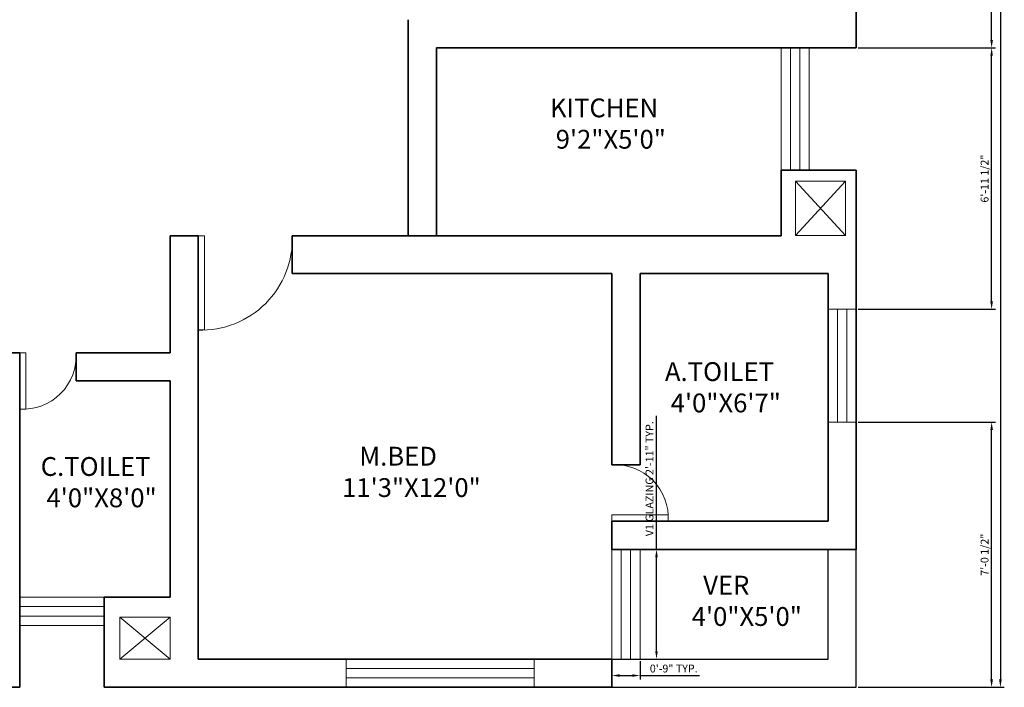
# Model space of a CAD drawing. Units: inches. Extents: x 3941 to 4852, y 2755 to 3388.
# Tile 4 of 5: x 4537 to 4852, y 2800 to 3013. Entities that reach past the tile are written whole.
import ezdxf

# ---------------------------------------------------------------- set-up
doc = ezdxf.new("R2010")
doc.units = ezdxf.units.IN
for name, color, linetype, lineweight in [('A-ANNO-DIMS', 2, 'Continuous', 18), ('A-AREA-IDEN', 7, 'Continuous', 18), ('A-DOOR', 2, 'Continuous', 18), ('A-FLOR-OPEN', 7, 'Continuous', 18), ('A-GLAZ', 5, 'Continuous', 18), ('A-WALL', 7, 'Continuous', 35), ('A-WALL-PRPT', 6, 'Continuous', 25)]:
    doc.layers.add(name, color=color, linetype=linetype, lineweight=lineweight)
doc.styles.get("Standard").update_dxf_attribs({"font": 'arial.ttf'})
doc.dimstyles.new('ISO-25', dxfattribs={"dimtxt": 2.5, "dimasz": 2.5, "dimexe": 1.25, "dimexo": 0.625, "dimtad": 1, "dimlunit": 3, "dimtxsty": 'Standard', "dimcen": 2.5, "dimadec": 0, "dimazin": 0, "dimtfac": 1, "dimtmove": 0, "dimatfit": 3, "dimfxl": 1, "dimarcsym": 0})

# ---------------------------------------------------------------- blocks, each defined once
blk = doc.blocks.new('*D2')
at = {"layer": 'A-ANNO-DIMS', "color": 0, "lineweight": -2, "transparency": 16777216}
for p, q in [((4804.88, 3327.75), (4851.51, 3327.75)), ((4850.26, 3325.25), (4850.26, 2802.25)), ((4804.88, 2799.75), (4851.51, 2799.75))]:
    blk.add_line(p, q, dxfattribs=at)
at = {"layer": 'A-ANNO-DIMS', "color": 0, "transparency": 16777216}
for points in [[(4849.85, 3325.25), (4850.68, 3325.25), (4850.26, 3327.75)], [(4849.85, 2802.25), (4850.68, 2802.25), (4850.26, 2799.75)]]:
    blk.add_solid(points, dxfattribs=at)
at = {"layer": 'Defpoints', "color": 0, "transparency": 16777216}
for p in [(4804.25, 3327.75), (4804.25, 2799.75), (4850.26, 2799.75)]:
    blk.add_point(p, dxfattribs=at)
at = {"layer": 'A-ANNO-DIMS', "color": 0, "transparency": 16777216, "insert": (4846.59, 3063.75), "char_height": 6, "attachment_point": 5, "rotation": 90}
blk.add_mtext('44\'-5"', dxfattribs=at)
blk = doc.blocks.new('WINDOW-60IN')
for p, q in [((0, 60), (9, 60)), ((0, 60), (0, 0)), ((3, 60), (3, 0)), ((6, 60), (6, 0)), ((9, 0), (9, 60)), ((0, 0), (9, 0))]:
    blk.add_line(p, q)
blk = doc.blocks.new('WINDOW-27IN')
for p, q in [((0, 0), (0, 27)), ((0, 27), (9, 27)), ((3, 0), (3, 27)), ((6, 0), (6, 27)), ((9, 27), (9, 0)), ((9, 0), (0, 0))]:
    blk.add_line(p, q)
blk = doc.blocks.new('WINDOW-36IN')
for p, q in [((0, 36), (9, 36)), ((0, 36), (0, 0)), ((3, 0), (3, 36)), ((6, 0), (6, 36)), ((9, 0), (9, 36)), ((0, 0), (9, 0))]:
    blk.add_line(p, q)
blk = doc.blocks.new('VERANDA-GLAZING-35IN')
for p, q in [((0, 35), (0, 0)), ((0, 35), (9, 35)), ((3, 35), (3, 0)), ((6, 35), (6, 0)), ((9, 35), (9, 0)), ((9, 35), (9, 0)), ((9, 0), (0, 0))]:
    blk.add_line(p, q)
blk = doc.blocks.new('DOOR-SWING-18IN')
for p, q in [((0.03, 0), (0.03, 2)), ((0.03, 2), (18.03, 2)), ((18.03, 0), (0.03, 0)), ((18.03, 2), (18.03, 0))]:
    blk.add_line(p, q)
blk.add_arc((17.03, 1), 17.03, 86.6335, 183.3665)
blk = doc.blocks.new('DOOR-SWING-30IN')
for p, q in [((0, 30.02), (30, 30.02)), ((0, 28.02), (0, 30.02)), ((30, 30.02), (30, 28.02)), ((30, 28.02), (0, 28.02))]:
    blk.add_line(p, q)
blk.add_arc((1, 29.02), 29.02, 268.0251, 1.9749)
blk = doc.blocks.new('*D25')
at = {"layer": 'A-ANNO-DIMS', "color": 0, "lineweight": -2, "transparency": 16777216}
for p, q in [((4740.5, 2843.75), (4740.5, 2886.36)), ((4735.88, 2843.75), (4741.75, 2843.75)), ((4740.5, 2811.25), (4740.5, 2841.25)), ((4735.88, 2808.75), (4741.75, 2808.75))]:
    blk.add_line(p, q, dxfattribs=at)
at = {"layer": 'A-ANNO-DIMS', "color": 0, "transparency": 16777216}
for points in [[(4740.09, 2841.25), (4740.92, 2841.25), (4740.5, 2843.75)], [(4740.09, 2811.25), (4740.92, 2811.25), (4740.5, 2808.75)]]:
    blk.add_solid(points, dxfattribs=at)
at = {"layer": 'Defpoints', "color": 0, "transparency": 16777216}
for p in [(4735.25, 2843.75), (4740.5, 2843.75), (4735.25, 2808.75)]:
    blk.add_point(p, dxfattribs=at)
at = {"layer": 'A-ANNO-DIMS', "color": 0, "transparency": 16777216, "insert": (4738.59, 2866.31), "char_height": 2.5, "attachment_point": 5, "rotation": 90}
blk.add_mtext('V1 GLAZING 2\'-11" TYP.', dxfattribs=at)
blk = doc.blocks.new('*D26')
at = {"layer": 'A-ANNO-DIMS', "color": 0, "lineweight": -2, "transparency": 16777216}
for p, q in [((4726.25, 2808.13), (4726.25, 2802.25)), ((4735.25, 2808.13), (4735.25, 2802.25)), ((4728.75, 2803.5), (4732.75, 2803.5)), ((4735.25, 2803.5), (4754.24, 2803.5))]:
    blk.add_line(p, q, dxfattribs=at)
at = {"layer": 'A-ANNO-DIMS', "color": 0, "transparency": 16777216}
for points in [[(4728.75, 2803.92), (4728.75, 2803.09), (4726.25, 2803.5)], [(4732.75, 2803.92), (4732.75, 2803.09), (4735.25, 2803.5)]]:
    blk.add_solid(points, dxfattribs=at)
at = {"layer": 'Defpoints', "color": 0, "transparency": 16777216}
for p in [(4726.25, 2808.75), (4735.25, 2808.75), (4735.25, 2803.5)]:
    blk.add_point(p, dxfattribs=at)
at = {"layer": 'A-ANNO-DIMS', "color": 0, "transparency": 16777216, "insert": (4746, 2805.41), "char_height": 2.5, "attachment_point": 5}
blk.add_mtext('0\'-9" TYP.', dxfattribs=at)
blk = doc.blocks.new('*D30')
at = {"layer": 'A-ANNO-DIMS', "color": 0, "lineweight": -2, "transparency": 16777216}
for p, q in [((4804.88, 2884.36), (4848.72, 2884.36)), ((4847.47, 2802.25), (4847.47, 2881.86)), ((4804.88, 2799.75), (4848.72, 2799.75))]:
    blk.add_line(p, q, dxfattribs=at)
at = {"layer": 'A-ANNO-DIMS', "color": 0, "transparency": 16777216}
for points in [[(4847.05, 2881.86), (4847.88, 2881.86), (4847.47, 2884.36)], [(4847.05, 2802.25), (4847.88, 2802.25), (4847.47, 2799.75)]]:
    blk.add_solid(points, dxfattribs=at)
at = {"layer": 'Defpoints', "color": 0, "transparency": 16777216}
for p in [(4804.25, 2884.36), (4847.47, 2884.36), (4804.25, 2799.75)]:
    blk.add_point(p, dxfattribs=at)
at = {"layer": 'A-ANNO-DIMS', "color": 0, "transparency": 16777216, "insert": (4845.55, 2842.06), "char_height": 2.5, "attachment_point": 5, "rotation": 90}
blk.add_mtext('7\'-0 1/2"', dxfattribs=at)
blk = doc.blocks.new('*D31')
at = {"layer": 'A-ANNO-DIMS', "color": 0, "lineweight": -2, "transparency": 16777216}
for p, q in [((4804.88, 3003.75), (4848.72, 3003.75)), ((4847.47, 2922.86), (4847.47, 3001.25)), ((4804.88, 2920.36), (4848.72, 2920.36))]:
    blk.add_line(p, q, dxfattribs=at)
at = {"layer": 'A-ANNO-DIMS', "color": 0, "transparency": 16777216}
for points in [[(4847.05, 3001.25), (4847.88, 3001.25), (4847.47, 3003.75)], [(4847.05, 2922.86), (4847.88, 2922.86), (4847.47, 2920.36)]]:
    blk.add_solid(points, dxfattribs=at)
at = {"layer": 'Defpoints', "color": 0, "transparency": 16777216}
for p in [(4804.25, 3003.75), (4847.47, 3003.75), (4804.25, 2920.36)]:
    blk.add_point(p, dxfattribs=at)
at = {"layer": 'A-ANNO-DIMS', "color": 0, "transparency": 16777216, "insert": (4845.55, 2962.06), "char_height": 2.5, "attachment_point": 5, "rotation": 90}
blk.add_mtext('6\'-11 1/2"', dxfattribs=at)
blk = doc.blocks.new('*D32')
at = {"layer": 'A-ANNO-DIMS', "color": 0, "lineweight": -2, "transparency": 16777216}
for p, q in [((4804.88, 3044.64), (4848.72, 3044.64)), ((4847.47, 3006.25), (4847.47, 3042.14)), ((4804.88, 3003.75), (4848.72, 3003.75))]:
    blk.add_line(p, q, dxfattribs=at)
at = {"layer": 'A-ANNO-DIMS', "color": 0, "transparency": 16777216}
for points in [[(4847.05, 3042.14), (4847.88, 3042.14), (4847.47, 3044.64)], [(4847.05, 3006.25), (4847.88, 3006.25), (4847.47, 3003.75)]]:
    blk.add_solid(points, dxfattribs=at)
at = {"layer": 'Defpoints', "color": 0, "transparency": 16777216}
for p in [(4804.25, 3044.64), (4847.47, 3044.64), (4804.25, 3003.75)]:
    blk.add_point(p, dxfattribs=at)
at = {"layer": 'A-ANNO-DIMS', "color": 0, "transparency": 16777216, "insert": (4845.56, 3024.2), "char_height": 2.5, "attachment_point": 5, "rotation": 90}
blk.add_mtext('3\'-5"', dxfattribs=at)

msp = doc.modelspace()

# ---------------------------------------------------------------- linework, layer by layer
at = {"layer": 'A-FLOR-OPEN'}
for p, q in [((4800.843, 2961.285), (4784.843, 2961.285)), ((4784.843, 2961.285), (4784.843, 2943.934)), ((4784.843, 2943.934), (4800.843, 2961.285)), ((4784.843, 2961.285), (4800.843, 2943.934)), ((4800.843, 2943.934), (4800.843, 2961.285)), ((4784.843, 2943.934), (4800.843, 2943.934)), ((4585.254, 2822.116), (4569.254, 2822.116)), ((4569.254, 2822.116), (4569.254, 2808.754)), ((4569.254, 2808.754), (4585.254, 2822.116)), ((4569.254, 2822.116), (4585.254, 2808.754)), ((4585.254, 2808.754), (4585.254, 2822.116)), ((4569.254, 2808.754), (4585.254, 2808.754))]:
    msp.add_line(p, q, dxfattribs=at)
at = {"layer": 'A-GLAZ'}
for p, q in [((4780.254, 3003.754), (4780.254, 2964.754)), ((4789.254, 3003.754), (4780.254, 3003.754)), ((4783.254, 3003.754), (4783.254, 2964.754)), ((4786.254, 3003.754), (4786.254, 2964.754)), ((4789.254, 2964.754), (4789.254, 3003.754)), ((4780.254, 2964.754), (4789.254, 2964.754))]:
    msp.add_line(p, q, dxfattribs=at)
at = {"layer": 'A-WALL'}
for p, q in [((4804.254, 3003.754), (4804.254, 3132.754)), ((4661.254, 3012.754), (4661.254, 2943.754)), ((4804.254, 3003.754), (4670.254, 3003.754)), ((4670.254, 3003.754), (4670.254, 2943.754)), ((4804.254, 2964.754), (4780.254, 2964.754)), ((4780.254, 2964.754), (4780.254, 2943.754)), ((4804.254, 2943.754), (4804.254, 2964.754)), ((4585.254, 2931.754), (4585.254, 2943.754)), ((4585.254, 2943.754), (4594.254, 2943.754)), ((4594.254, 2943.754), (4594.254, 2897.492)), ((4780.254, 2943.754), (4624.254, 2943.754)), ((4624.254, 2943.754), (4624.254, 2931.754)), ((4804.254, 2843.754), (4804.254, 2943.754)), ((4585.254, 2931.754), (4585.254, 2906.492)), ((4624.254, 2931.754), (4726.254, 2931.754)), ((4726.254, 2870.754), (4726.254, 2931.754)), ((4735.254, 2931.754), (4795.254, 2931.754)), ((4735.254, 2870.754), (4735.254, 2931.754)), ((4795.254, 2852.754), (4795.254, 2931.754)), ((4528.254, 2906.492), (4537.254, 2906.492)), ((4537.254, 2906.492), (4537.254, 2897.492)), ((4585.254, 2906.492), (4555.254, 2906.492)), ((4555.254, 2906.492), (4555.254, 2897.492)), ((4537.254, 2799.754), (4537.254, 2897.492)), ((4585.254, 2897.492), (4555.254, 2897.492)), ((4585.254, 2828.492), (4585.254, 2897.492)), ((4594.254, 2808.754), (4594.254, 2897.492)), ((4726.254, 2870.754), (4735.254, 2870.754)), ((4726.254, 2852.754), (4795.254, 2852.754)), ((4726.254, 2843.754), (4726.254, 2852.754)), ((4726.254, 2843.754), (4804.254, 2843.754)), ((4585.254, 2828.492), (4564.254, 2828.492)), ((4564.254, 2828.492), (4564.254, 2799.754)), ((4726.254, 2808.754), (4594.254, 2808.754)), ((4726.254, 2799.754), (4726.254, 2808.754)), ((4537.254, 2799.754), (4246.254, 2799.754)), ((4564.254, 2799.754), (4585.254, 2799.754)), ((4726.254, 2799.754), (4585.254, 2799.754))]:
    msp.add_line(p, q, dxfattribs=at)
at = {"layer": 'A-WALL-PRPT'}
for p, q in [((4795.254, 2808.754), (4795.254, 2843.754)), ((4804.254, 2799.754), (4804.254, 2843.754)), ((4726.254, 2808.754), (4795.254, 2808.754)), ((4726.254, 2799.754), (4804.254, 2799.754))]:
    msp.add_line(p, q, dxfattribs=at)

# ---------------------------------------------------------------- block references
at = {"layer": 'A-DOOR', "extrusion": (0, 0, -1), "zscale": -1}
for name, p, rotation in [('DOOR-SWING-30IN', (-4624.27, 2943.754), 270.0000000000027), ('DOOR-SWING-18IN', (-4537.253, 2888.462), 90.00000000000261)]:
    msp.add_blockref(name, p, dxfattribs=dict(at, rotation=rotation))
msp.add_blockref('DOOR-SWING-18IN', (-4744.283, 2852.754), dxfattribs=at)
at = {"layer": 'A-GLAZ'}
for name, p, rotation in [('WINDOW-36IN', (4804.253, 2920.365), 180), ('WINDOW-27IN', (4537.253, 2828.492), 270.0000000000023), ('WINDOW-60IN', (4701.479, 2799.755), 89.99999999999947)]:
    msp.add_blockref(name, p, dxfattribs=dict(at, rotation=rotation))
msp.add_blockref('VERANDA-GLAZING-35IN', (4726.254, 2808.754), dxfattribs=at)

# ---------------------------------------------------------------- texts
at = {"layer": 'A-AREA-IDEN', "char_height": 6, "attachment_point": 1}
for s, insert in [(' KITCHEN\\P  9\'2"X5\'0"', (4704.672, 2987.611)), ('A.TOILET\\P 4\'0"X6\'7"', (4743.203, 2903.478)), ('    M.BED\\P 11\'3"X12\'0"', (4638.326, 2876.478)), (' C.TOILET\\P  4\'0"X8\'0"', (4542.134, 2873.203)), ('  VER\\P4\'0"X5\'0"', (4751.746, 2835.343))]:
    msp.add_mtext_dynamic_manual_height_columns(s, width=69.57529, gutter_width=12.5, heights=[0], dxfattribs=dict(at, insert=insert))

# ---------------------------------------------------------------- dimensions: what is measured, and where the dimension line sits
at = {"layer": 'A-ANNO-DIMS'}
for base, p1, p2, text, override, picture, middle in [((4850.264, 2799.754), (4804.254, 3327.754), (4804.254, 2799.754), '<>-5"', {"dimtxt": 6, "dimclrd": 0, "dimclre": 0, "dimclrt": 0}, '*D2', (4846.588, 3063.754)), ((4740.504, 2843.754), (4735.254, 2808.754), (4735.254, 2843.754), 'V1 GLAZING <> TYP.', {"dimdec": 1, "dimlfac": 1, "dimrnd": 0, "dimzin": 1, "dimdsep": 46, "dimlunit": 4, "dimfrac": 2}, '*D25', (4738.586, 2866.306))]:
    dim = msp.add_linear_dim(base=base, p1=p1, p2=p2, angle=90, text=text, dimstyle='ISO-25', override=override, dxfattribs=at)
    dim.commit()
    dim.dimension.update_dxf_attribs({"geometry": picture, "text_midpoint": middle})
for base, p1, p2, picture, middle in [((4847.466, 3044.641), (4804.254, 3003.754), (4804.254, 3044.641), '*D32', (4845.564, 3024.198)), ((4847.466, 3003.754), (4804.254, 2920.365), (4804.254, 3003.754), '*D31', (4845.549, 2962.06)), ((4847.466, 2884.365), (4804.254, 2799.754), (4804.254, 2884.365), '*D30', (4845.549, 2842.06))]:
    dim = msp.add_linear_dim(base=base, p1=p1, p2=p2, angle=90, dimstyle='ISO-25', override={"dimdec": 1, "dimlfac": 1, "dimrnd": 0, "dimzin": 1, "dimdsep": 46, "dimlunit": 4, "dimfrac": 2}, dxfattribs=at)
    dim.commit()
    dim.dimension.update_dxf_attribs({"geometry": picture, "text_midpoint": middle})
dim = msp.add_linear_dim(base=(4735.254, 2803.504), p1=(4726.254, 2808.754), p2=(4735.254, 2808.754), text='<> TYP.', dimstyle='ISO-25', override={"dimdec": 1, "dimlfac": 1, "dimrnd": 0, "dimzin": 1, "dimdsep": 46, "dimlunit": 4, "dimfrac": 2}, dxfattribs=at)
dim.commit()
dim.dimension.update_dxf_attribs({"geometry": '*D26', "text_midpoint": (4745.998, 2805.406)})

doc.saveas('drawing.dxf')
